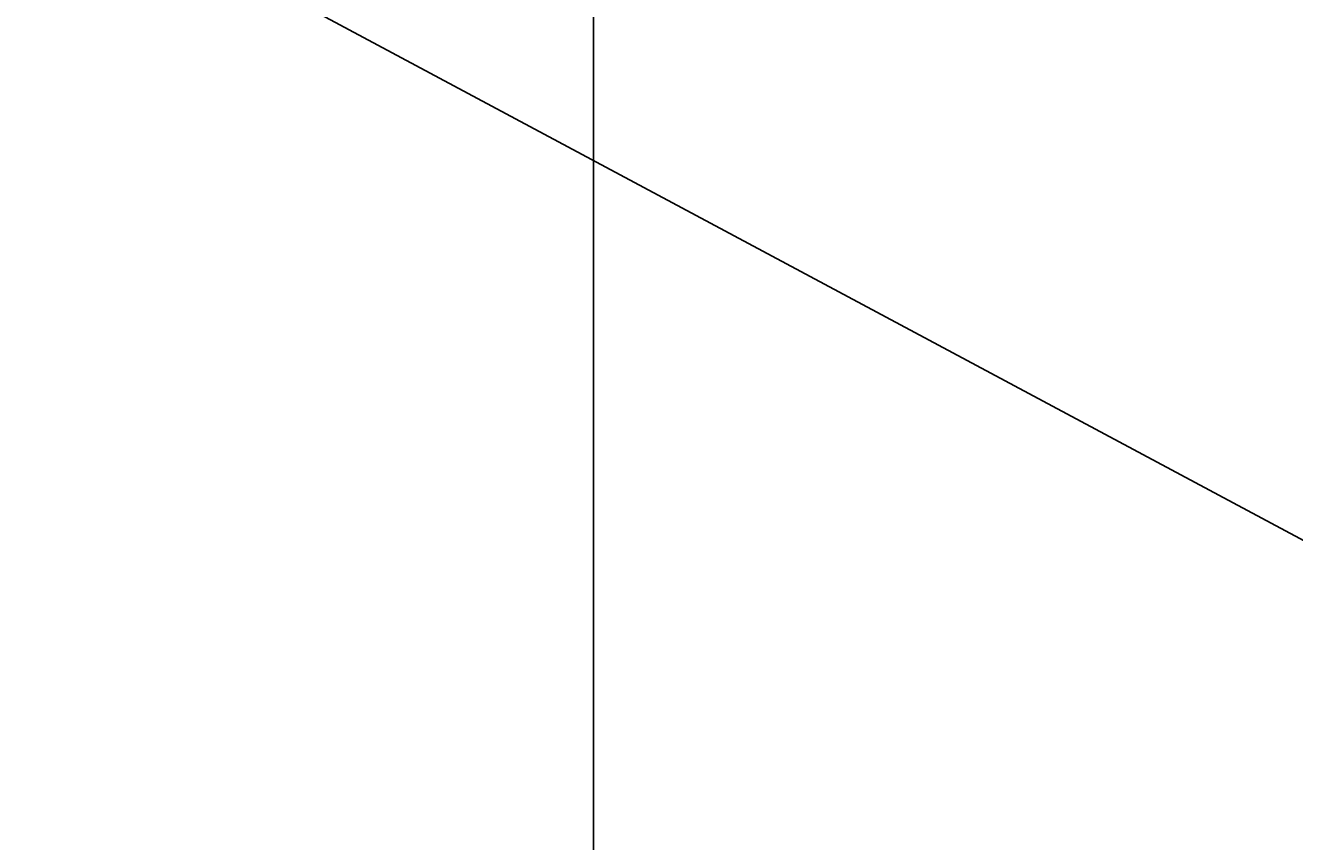
# Model space of a CAD drawing. Units: inches. Extents: x 35362 to 73946, y 43607 to 67532.
# Tile 115 of 134: x 51013 to 51049, y 49038 to 49061. Entities that reach past the tile are written whole.
import ezdxf

# ---------------------------------------------------------------- set-up
doc = ezdxf.new("R2010")
doc.units = ezdxf.units.IN
doc.header["$MEASUREMENT"] = 0
doc.layers.add('A-ANNO-DIMS', color=2, linetype='Continuous', lineweight=18)
doc.layers.add('E-SYMB', color=1, linetype='Continuous', lineweight=25)
doc.styles.get("Standard").update_dxf_attribs({"font": 'arial.ttf'})
doc.dimstyles.get("Standard").update_dxf_attribs({"dimtxt": 0.18, "dimasz": 0.18, "dimexe": 0.18, "dimexo": 0.0625, "dimgap": 0.09, "dimtad": 0, "dimtih": 1, "dimtoh": 1, "dimdec": 4, "dimzin": 0, "dimdsep": 46, "dimtxsty": 'Standard', "dimcen": 0.09, "dimadec": 0, "dimazin": 0, "dimtfac": 1, "dimtdec": 4, "dimtofl": 0, "dimtmove": 0, "dimatfit": 3, "dimfxl": 1, "dimtolj": 1, "dimtzin": 0, "dimarcsym": 0})

# ---------------------------------------------------------------- blocks, each defined once
blk = doc.blocks.new('*D11')
at = {"layer": 'A-ANNO-DIMS', "color": 0, "lineweight": -2, "transparency": 16777216}
for p, q in [((47978.665, 56028.774), (47978.665, 43606.679)), ((53109.76, 56028.774), (53109.76, 43606.679)), ((47978.845, 43606.859), (50543.871, 43606.859)), ((53109.58, 43606.859), (50544.554, 43606.859))]:
    blk.add_line(p, q, dxfattribs=at)
at = {"layer": 'A-ANNO-DIMS', "color": 0, "transparency": 16777216}
for points in [[(47978.845, 43606.889), (47978.845, 43606.829), (47978.665, 43606.859)], [(53109.58, 43606.889), (53109.58, 43606.829), (53109.76, 43606.859)]]:
    blk.add_solid(points, dxfattribs=at)
at = {"layer": 'Defpoints', "color": 0, "transparency": 16777216}
for p in [(47978.665, 56028.836), (53109.76, 56028.836), (53109.76, 43606.859)]:
    blk.add_point(p, dxfattribs=at)
at = {"layer": 'A-ANNO-DIMS', "color": 0, "transparency": 16777216, "insert": (50544.212, 43606.859), "char_height": 0.18, "attachment_point": 5}
blk.add_mtext('\\A1;5131', dxfattribs=at)
blk = doc.blocks.new('*D13')
at = {"layer": 'A-ANNO-DIMS', "color": 0, "lineweight": -2, "transparency": 16777216}
for p, q in [((48373.492, 51694.025), (48373.492, 43606.679)), ((51029.043, 51694.025), (51029.043, 43606.679)), ((48373.672, 43606.859), (49700.802, 43606.859)), ((51028.863, 43606.859), (49701.733, 43606.859))]:
    blk.add_line(p, q, dxfattribs=at)
at = {"layer": 'A-ANNO-DIMS', "color": 0, "transparency": 16777216}
for points in [[(48373.672, 43606.889), (48373.672, 43606.829), (48373.492, 43606.859)], [(51028.863, 43606.889), (51028.863, 43606.829), (51029.043, 43606.859)]]:
    blk.add_solid(points, dxfattribs=at)
at = {"layer": 'Defpoints', "color": 0, "transparency": 16777216}
for p in [(48373.492, 51694.087), (51029.043, 51694.087), (51029.043, 43606.859)]:
    blk.add_point(p, dxfattribs=at)
at = {"layer": 'A-ANNO-DIMS', "color": 0, "transparency": 16777216, "insert": (49701.267, 43606.859), "char_height": 0.18, "attachment_point": 5}
blk.add_mtext('\\A1;2655.6', dxfattribs=at)
blk = doc.blocks.new('*D17')
at = {"layer": 'A-ANNO-DIMS', "color": 0, "lineweight": -2, "transparency": 16777216}
for p, q in [((49923.307, 61293.224), (49923.307, 43606.679)), ((51913.931, 61293.224), (51913.931, 43606.679)), ((49923.487, 43606.859), (50918.164, 43606.859)), ((51913.751, 43606.859), (50919.074, 43606.859))]:
    blk.add_line(p, q, dxfattribs=at)
at = {"layer": 'A-ANNO-DIMS', "color": 0, "transparency": 16777216}
for points in [[(49923.487, 43606.889), (49923.487, 43606.829), (49923.307, 43606.859)], [(51913.751, 43606.889), (51913.751, 43606.829), (51913.931, 43606.859)]]:
    blk.add_solid(points, dxfattribs=at)
at = {"layer": 'Defpoints', "color": 0, "transparency": 16777216}
for p in [(49923.307, 61293.286), (51913.931, 61293.286), (51913.931, 43606.859)]:
    blk.add_point(p, dxfattribs=at)
at = {"layer": 'A-ANNO-DIMS', "color": 0, "transparency": 16777216, "insert": (50918.619, 43606.859), "char_height": 0.18, "attachment_point": 5}
blk.add_mtext('\\A1;1990.6', dxfattribs=at)
blk = doc.blocks.new('*D67')
at = {"layer": 'A-ANNO-DIMS', "color": 0, "lineweight": -2, "transparency": 16777216}
for p, q in [((56873.539, 53351.529), (35361.769, 53351.529)), ((35361.949, 53351.349), (35361.949, 49400.893)), ((35361.949, 45450.074), (35361.949, 49400.53)), ((53793.575, 45449.894), (35361.769, 45449.894))]:
    blk.add_line(p, q, dxfattribs=at)
at = {"layer": 'A-ANNO-DIMS', "color": 0, "transparency": 16777216}
for points in [[(35361.919, 53351.349), (35361.979, 53351.349), (35361.949, 53351.529)], [(35361.919, 45450.074), (35361.979, 45450.074), (35361.949, 45449.894)]]:
    blk.add_solid(points, dxfattribs=at)
at = {"layer": 'Defpoints', "color": 0, "transparency": 16777216}
for p in [(35361.949, 53351.529), (56873.602, 53351.529), (53793.638, 45449.894)]:
    blk.add_point(p, dxfattribs=at)
at = {"layer": 'A-ANNO-DIMS', "color": 0, "transparency": 16777216, "insert": (35361.949, 49400.712), "char_height": 0.18, "attachment_point": 5}
blk.add_mtext('\\A1;7901.6', dxfattribs=at)
blk = doc.blocks.new('*D84')
at = {"layer": 'A-ANNO-DIMS', "color": 0, "lineweight": -2, "transparency": 16777216}
for p, q in [((55540.235, 49259.935), (35361.769, 49259.935)), ((35361.949, 49259.755), (35361.949, 49115.139)), ((35361.949, 48970.16), (35361.949, 49114.776)), ((55540.235, 48969.98), (35361.769, 48969.98))]:
    blk.add_line(p, q, dxfattribs=at)
at = {"layer": 'A-ANNO-DIMS', "color": 0, "transparency": 16777216}
for points in [[(35361.919, 49259.755), (35361.979, 49259.755), (35361.949, 49259.935)], [(35361.919, 48970.16), (35361.979, 48970.16), (35361.949, 48969.98)]]:
    blk.add_solid(points, dxfattribs=at)
at = {"layer": 'Defpoints', "color": 0, "transparency": 16777216}
for p in [(35361.949, 49259.935), (55540.297, 49259.935), (55540.297, 48969.98)]:
    blk.add_point(p, dxfattribs=at)
at = {"layer": 'A-ANNO-DIMS', "color": 0, "transparency": 16777216, "insert": (35361.949, 49114.957), "char_height": 0.18, "attachment_point": 5}
blk.add_mtext('\\A1;289.96', dxfattribs=at)
blk = doc.blocks.new('*D86')
at = {"layer": 'A-ANNO-DIMS', "color": 0, "lineweight": -2, "transparency": 16777216}
for p, q in [((51285.532, 49320.079), (35361.769, 49320.079)), ((35361.949, 49319.899), (35361.949, 49120.261)), ((35361.949, 48920.259), (35361.949, 49119.897)), ((51285.532, 48920.079), (35361.769, 48920.079))]:
    blk.add_line(p, q, dxfattribs=at)
at = {"layer": 'A-ANNO-DIMS', "color": 0, "transparency": 16777216}
for points in [[(35361.919, 49319.899), (35361.979, 49319.899), (35361.949, 49320.079)], [(35361.919, 48920.259), (35361.979, 48920.259), (35361.949, 48920.079)]]:
    blk.add_solid(points, dxfattribs=at)
at = {"layer": 'Defpoints', "color": 0, "transparency": 16777216}
for p in [(35361.949, 49320.079), (51285.595, 49320.079), (51285.595, 48920.079)]:
    blk.add_point(p, dxfattribs=at)
at = {"layer": 'A-ANNO-DIMS', "color": 0, "transparency": 16777216, "insert": (35361.949, 49120.079), "char_height": 0.18, "attachment_point": 5}
blk.add_mtext('\\A1;400.0', dxfattribs=at)
blk = doc.blocks.new('*D107')
at = {"layer": 'A-ANNO-DIMS', "color": 0, "lineweight": -2, "transparency": 16777216}
for p, q in [((50139.563, 59850.014), (50139.563, 43606.679)), ((51320.813, 59850.014), (51320.813, 43606.679)), ((50139.743, 43606.859), (50729.733, 43606.859)), ((51320.633, 43606.859), (50730.643, 43606.859))]:
    blk.add_line(p, q, dxfattribs=at)
at = {"layer": 'A-ANNO-DIMS', "color": 0, "transparency": 16777216}
for points in [[(50139.743, 43606.889), (50139.743, 43606.829), (50139.563, 43606.859)], [(51320.633, 43606.889), (51320.633, 43606.829), (51320.813, 43606.859)]]:
    blk.add_solid(points, dxfattribs=at)
at = {"layer": 'Defpoints', "color": 0, "transparency": 16777216}
for p in [(50139.563, 59850.077), (51320.813, 59850.077), (51320.813, 43606.859)]:
    blk.add_point(p, dxfattribs=at)
at = {"layer": 'A-ANNO-DIMS', "color": 0, "transparency": 16777216, "insert": (50730.188, 43606.859), "char_height": 0.18, "attachment_point": 5}
blk.add_mtext('\\A1;1181.3', dxfattribs=at)

msp = doc.modelspace()

# ---------------------------------------------------------------- linework, layer by layer
at = {"layer": 'E-SYMB'}
msp.add_line((50952.662, 49098.368), (51285.595, 48920.079), dxfattribs=at)

# ---------------------------------------------------------------- dimensions: what is measured, and where the dimension line sits
at = {"layer": 'A-ANNO-DIMS'}
for base, p1, p2, override, picture, middle in [((51913.931, 43606.859), (49923.307, 61293.286), (51913.931, 61293.286), {"dimdec": 1, "dimlfac": 1, "dimrnd": 0, "dimzin": 0, "dimdsep": 46, "dimlunit": 2}, '*D17', (50918.619, 43606.859)), ((51320.8133, 43606.859), (50139.5627, 59850.0769), (51320.8133, 59850.0769), {"dimdec": 1, "dimlfac": 1, "dimrnd": 0, "dimzin": 0, "dimdsep": 46, "dimlunit": 2}, '*D107', (50730.188, 43606.859)), ((53109.76, 43606.859), (47978.665, 56028.836), (53109.76, 56028.836), {"dimdec": 0, "dimlfac": 1, "dimrnd": 0, "dimzin": 0, "dimdsep": 46, "dimlunit": 2}, '*D11', (50544.212, 43606.859)), ((51029.043, 43606.859), (48373.492, 51694.087), (51029.043, 51694.087), {"dimdec": 1, "dimlfac": 1, "dimrnd": 0, "dimzin": 0, "dimdsep": 46, "dimlunit": 2}, '*D13', (49701.267, 43606.859))]:
    dim = msp.add_linear_dim(base=base, p1=p1, p2=p2, dimstyle='Standard', override=override, dxfattribs=at)
    dim.commit()
    dim.dimension.update_dxf_attribs({"geometry": picture, "text_midpoint": middle})
for base, p1, p2, override, picture, middle in [((35361.949, 53351.529), (53793.638, 45449.894), (56873.602, 53351.529), {"dimdec": 1, "dimlfac": 1, "dimrnd": 0, "dimzin": 0, "dimdsep": 46, "dimlunit": 2}, '*D67', (35361.949, 49400.712)), ((35361.949, 49320.079), (51285.595, 48920.079), (51285.595, 49320.079), {"dimdec": 1, "dimlfac": 1, "dimrnd": 0, "dimzin": 0, "dimdsep": 46, "dimlunit": 2}, '*D86', (35361.949, 49120.079)), ((35361.9491, 49259.9353), (55540.2972, 48969.9796), (55540.2972, 49259.9353), {"dimdec": 2, "dimlfac": 1, "dimrnd": 0, "dimzin": 0, "dimdsep": 46, "dimlunit": 2}, '*D84', (35361.9491, 49114.9575))]:
    dim = msp.add_linear_dim(base=base, p1=p1, p2=p2, angle=90, dimstyle='Standard', override=override, dxfattribs=at)
    dim.commit()
    dim.dimension.update_dxf_attribs({"geometry": picture, "text_midpoint": middle})

doc.saveas('drawing.dxf')
